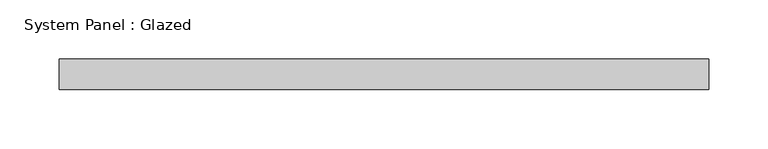
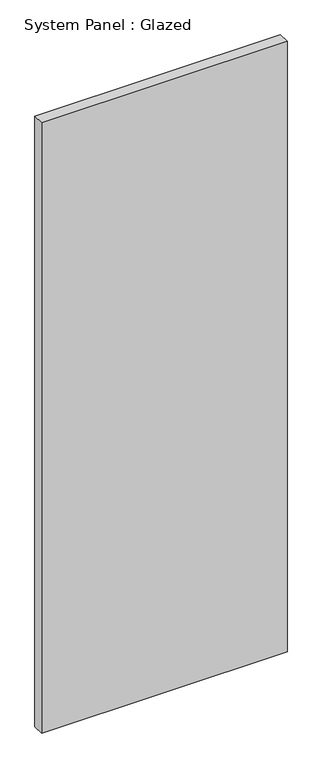
"""IFC4 building model written with IfcOpenShell, lengths in millimetres: plate geometry, System Panel : Glazed."""

from ifc_helpers import new_model, si_unit, origin, origin_with_axes, place, context, project, spatial, polyline, outline, extrude, source, transform, mapped, element, save


def system_panel_glazed_74412268(model_context):
    return source(origin(), model_context, "Body", "SweptSolid", [
        extrude(outline(polyline([(273.05, 19.05), (-273.05, 19.05), (-273.05, 44.45), (273.05, 44.45), (273.05, 19.05)])), origin_with_axes(), (0.0, 0.0, 1.0), 1435.1313909),
    ])


if __name__ == "__main__":
    model = new_model("IFC4")
    model_context = context("Model", 3, world=origin())
    ifc_project = project(units=[si_unit("LENGTHUNIT", "METRE", prefix="MILLI")], contexts=[model_context])
    site = spatial("IfcSite", under=ifc_project)
    building = spatial("IfcBuilding", under=site)
    placement = place(None, origin())
    system_panel_glazed_shape = system_panel_glazed_74412268(model_context)
    element("IfcPlate", 1, ObjectType="System Panel : Glazed", at=placement, inside=building, context=model_context, shape_type="MappedRepresentation", body=[
        mapped(system_panel_glazed_shape, transform((0.0, 0.0, 0.0), x_axis=(1.0, 0.0, 0.0), y_axis=(0.0, 1.0, 0.0), z_axis=(0.0, 0.0, 1.0))),
    ])
    save(model, "model.ifc")

# Revit data of these elements
# Type "System Panel : Glazed"
#   Construction Type Id = "GSP4R"
#   Analytic Construction = "1/8 in Pilkington single glazing"
#   Visual Light Transmittance = 0.9
#   Solar Heat Gain Coefficient = 0.86
#   Heat Transfer Coefficient (U) = 1.18115 BTU/(h·ft²·°F)
#   Define Thermal Properties by = 1
# Element 1 (IfcPlate, "System Panel : Glazed")
#   Materials on its faces: "Glass"
# Materials
#   "Glass": class "Glass", colour RGB 0 128 192, transparency 0.75, Description = "Soda Lime Glass", Cost = 0
